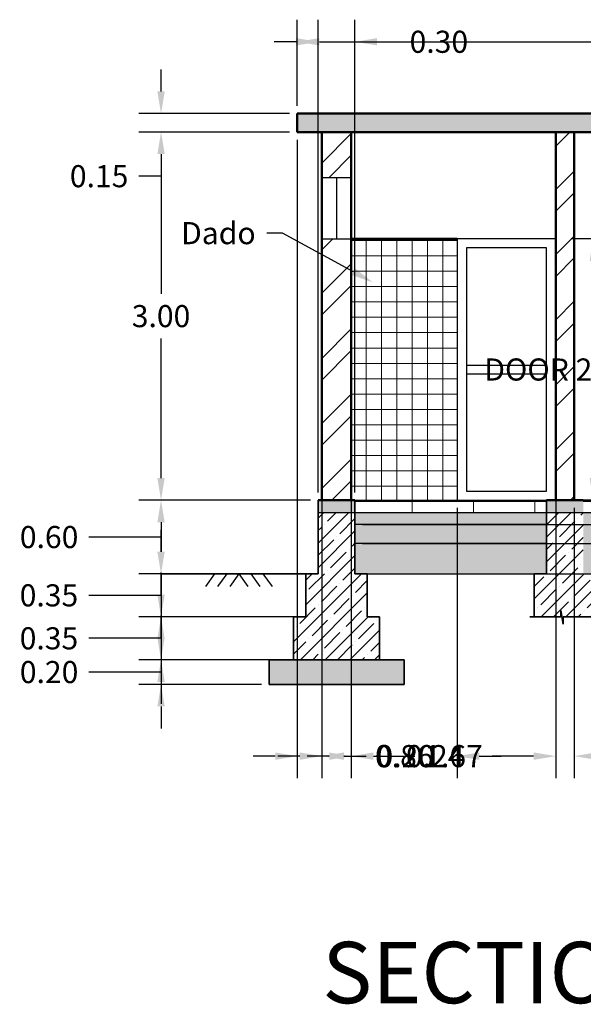
# Model space of a CAD drawing. Units: metres. Extents: x 22.1 to 34.4, y 4.4 to 12.4.
# Tile 1 of 8: x 22.1 to 26.6, y 4.4 to 12.4. Entities that reach past the tile are written whole.
import ezdxf
from ezdxf import colors
from ezdxf.entities.mleader import LeaderData, LeaderLine
from ezdxf.math import Vec2, Vec3

# ---------------------------------------------------------------- set-up
doc = ezdxf.new("R2010")
doc.units = ezdxf.units.M
doc.header["$MEASUREMENT"] = 0
for name, color, linetype, lineweight in [('A-ANNO-DIMS', 2, 'Continuous', 18), ('A-ANNO-TEXT', 7, 'Continuous', 18), ('A-DOOR', 4, 'Continuous', 25), ('A-FLOR', 3, 'Continuous', 25), ('A-FLOR-PATT', 252, 'Continuous', 13), ('A-GLAZ', 4, 'Continuous', 25), ('A-WALL', 7, 'Continuous', 50), ('A-WALL-PATT', 8, 'Continuous', 18), ('C-TOPO', 3, 'Continuous', 25), ('S-FNDN', 1, 'Continuous', 35), ('S-FNDN-PATT', 8, 'Continuous', 13), ('S-SLAB', 1, 'Continuous', 50), ('S-SLAB-PATT', 8, 'Continuous', 13)]:
    doc.layers.add(name, color=color, linetype=linetype, lineweight=lineweight)
doc.styles.get("Standard").update_dxf_attribs({"font": 'arial.ttf'})
doc.dimstyles.get("Standard").update_dxf_attribs({"dimtxt": 0.18, "dimasz": 0.18, "dimexe": 0.18, "dimexo": 0.0625, "dimgap": 0.09, "dimtad": 0, "dimtih": 1, "dimtoh": 1, "dimzin": 0, "dimdsep": 46, "dimtxsty": 'Standard', "dimcen": 0.09, "dimadec": 0, "dimazin": 0, "dimtfac": 1, "dimtofl": 0, "dimtmove": 0, "dimatfit": 3, "dimfxl": 1, "dimtolj": 1, "dimtzin": 0, "dimarcsym": 0})

# ---------------------------------------------------------------- blocks, each defined once
blk = doc.blocks.new('*D1')
at = {"layer": 'A-ANNO-DIMS', "color": 0, "lineweight": -2, "transparency": 16777216}
for p, q in [((23.2043, 11.8399), (23.2043, 12.0199)), ((24.2524, 11.6599), (23.0243, 11.6599)), ((24.2524, 11.5099), (23.0243, 11.5099)), ((23.2043, 11.3299), (23.2043, 11.1499)), ((23.2043, 11.1499), (23.0243, 11.1499))]:
    blk.add_line(p, q, dxfattribs=at)
at = {"layer": 'A-ANNO-DIMS', "color": 0, "transparency": 16777216}
for points in [[(23.1743, 11.8399), (23.2343, 11.8399), (23.2043, 11.6599)], [(23.1743, 11.3299), (23.2343, 11.3299), (23.2043, 11.5099)]]:
    blk.add_solid(points, dxfattribs=at)
at = {"layer": 'Defpoints', "color": 0, "transparency": 16777216}
for p in [(24.3149, 11.6599), (23.2043, 11.5099), (24.3149, 11.5099)]:
    blk.add_point(p, dxfattribs=at)
at = {"layer": 'A-ANNO-DIMS', "color": 0, "transparency": 16777216, "insert": (22.6998, 11.1499), "char_height": 0.18, "attachment_point": 5}
blk.add_mtext('\\A1;0.15', dxfattribs=at)
blk = doc.blocks.new('*D2')
at = {"layer": 'A-ANNO-DIMS', "color": 0, "lineweight": -2, "transparency": 16777216}
for p, q in [((24.2524, 11.5099), (23.0243, 11.5099)), ((23.2043, 11.3299), (23.2043, 10.1919)), ((23.2043, 8.6899), (23.2043, 9.8279)), ((24.4224, 8.5099), (23.0243, 8.5099))]:
    blk.add_line(p, q, dxfattribs=at)
at = {"layer": 'A-ANNO-DIMS', "color": 0, "transparency": 16777216}
for points in [[(23.1743, 11.3299), (23.2343, 11.3299), (23.2043, 11.5099)], [(23.1743, 8.6899), (23.2343, 8.6899), (23.2043, 8.5099)]]:
    blk.add_solid(points, dxfattribs=at)
at = {"layer": 'Defpoints', "color": 0, "transparency": 16777216}
for p in [(24.3149, 11.5099), (23.2043, 8.5099), (24.4849, 8.5099)]:
    blk.add_point(p, dxfattribs=at)
at = {"layer": 'A-ANNO-DIMS', "color": 0, "transparency": 16777216, "insert": (23.2043, 10.0099), "char_height": 0.18, "attachment_point": 5}
blk.add_mtext('\\A1;3.00', dxfattribs=at)
blk = doc.blocks.new('*D3')
at = {"layer": 'A-ANNO-DIMS', "color": 0, "lineweight": -2, "transparency": 16777216}
for p, q in [((24.4224, 8.5099), (23.0243, 8.5099)), ((23.2043, 8.3299), (23.2043, 8.0899)), ((22.7955, 8.2099), (22.6155, 8.2099)), ((23.2043, 8.2099), (22.7955, 8.2099)), ((24.4224, 7.9099), (23.0243, 7.9099))]:
    blk.add_line(p, q, dxfattribs=at)
at = {"layer": 'A-ANNO-DIMS', "color": 0, "transparency": 16777216}
for points in [[(23.1743, 8.3299), (23.2343, 8.3299), (23.2043, 8.5099)], [(23.1743, 8.0899), (23.2343, 8.0899), (23.2043, 7.9099)]]:
    blk.add_solid(points, dxfattribs=at)
at = {"layer": 'Defpoints', "color": 0, "transparency": 16777216}
for p in [(24.4849, 8.5099), (23.2043, 7.9099), (24.4849, 7.9099)]:
    blk.add_point(p, dxfattribs=at)
at = {"layer": 'A-ANNO-DIMS', "color": 0, "transparency": 16777216, "insert": (22.292, 8.2099), "char_height": 0.18, "attachment_point": 5}
blk.add_mtext('\\A1;0.60', dxfattribs=at)
blk = doc.blocks.new('*D4')
at = {"layer": 'A-ANNO-DIMS', "color": 0, "lineweight": -2, "transparency": 16777216}
for p, q in [((23.2043, 8.0899), (23.2043, 8.2699)), ((24.4224, 7.9099), (23.0243, 7.9099)), ((23.2043, 7.9099), (23.2043, 7.5599)), ((22.7954, 7.7349), (22.6154, 7.7349)), ((23.2043, 7.7349), (22.7954, 7.7349)), ((24.3224, 7.5599), (23.0243, 7.5599)), ((23.2043, 7.3799), (23.2043, 7.1999))]:
    blk.add_line(p, q, dxfattribs=at)
at = {"layer": 'A-ANNO-DIMS', "color": 0, "transparency": 16777216}
for points in [[(23.1743, 8.0899), (23.2343, 8.0899), (23.2043, 7.9099)], [(23.1743, 7.3799), (23.2343, 7.3799), (23.2043, 7.5599)]]:
    blk.add_solid(points, dxfattribs=at)
at = {"layer": 'Defpoints', "color": 0, "transparency": 16777216}
for p in [(24.4849, 7.9099), (23.2043, 7.5599), (24.3849, 7.5599)]:
    blk.add_point(p, dxfattribs=at)
at = {"layer": 'A-ANNO-DIMS', "color": 0, "transparency": 16777216, "insert": (22.2909, 7.7349), "char_height": 0.18, "attachment_point": 5}
blk.add_mtext('\\A1;0.35', dxfattribs=at)
blk = doc.blocks.new('*D5')
at = {"layer": 'A-ANNO-DIMS', "color": 0, "lineweight": -2, "transparency": 16777216}
for p, q in [((23.2043, 7.7399), (23.2043, 7.9199)), ((24.3224, 7.5599), (23.0243, 7.5599)), ((23.2043, 7.5599), (23.2043, 7.2099)), ((22.7954, 7.3849), (22.6154, 7.3849)), ((23.2043, 7.3849), (22.7954, 7.3849)), ((24.2224, 7.2099), (23.0243, 7.2099)), ((23.2043, 7.0299), (23.2043, 6.8499))]:
    blk.add_line(p, q, dxfattribs=at)
at = {"layer": 'A-ANNO-DIMS', "color": 0, "transparency": 16777216}
for points in [[(23.1743, 7.7399), (23.2343, 7.7399), (23.2043, 7.5599)], [(23.1743, 7.0299), (23.2343, 7.0299), (23.2043, 7.2099)]]:
    blk.add_solid(points, dxfattribs=at)
at = {"layer": 'Defpoints', "color": 0, "transparency": 16777216}
for p in [(24.3849, 7.5599), (23.2043, 7.2099), (24.2849, 7.2099)]:
    blk.add_point(p, dxfattribs=at)
at = {"layer": 'A-ANNO-DIMS', "color": 0, "transparency": 16777216, "insert": (22.2909, 7.3849), "char_height": 0.18, "attachment_point": 5}
blk.add_mtext('\\A1;0.35', dxfattribs=at)
blk = doc.blocks.new('*D6')
at = {"layer": 'A-ANNO-DIMS', "color": 0, "lineweight": -2, "transparency": 16777216}
for p, q in [((23.2043, 7.3899), (23.2043, 7.5699)), ((24.2224, 7.2099), (23.0243, 7.2099)), ((23.2043, 7.2099), (23.2043, 7.0099)), ((22.7955, 7.1099), (22.6155, 7.1099)), ((23.2043, 7.1099), (22.7955, 7.1099)), ((24.0224, 7.0099), (23.0243, 7.0099)), ((23.2043, 6.8299), (23.2043, 6.6499))]:
    blk.add_line(p, q, dxfattribs=at)
at = {"layer": 'A-ANNO-DIMS', "color": 0, "transparency": 16777216}
for points in [[(23.1743, 7.3899), (23.2343, 7.3899), (23.2043, 7.2099)], [(23.1743, 6.8299), (23.2343, 6.8299), (23.2043, 7.0099)]]:
    blk.add_solid(points, dxfattribs=at)
at = {"layer": 'Defpoints', "color": 0, "transparency": 16777216}
for p in [(24.2849, 7.2099), (23.2043, 7.0099), (24.0849, 7.0099)]:
    blk.add_point(p, dxfattribs=at)
at = {"layer": 'A-ANNO-DIMS', "color": 0, "transparency": 16777216, "insert": (22.292, 7.1099), "char_height": 0.18, "attachment_point": 5}
blk.add_mtext('\\A1;0.20', dxfattribs=at)
blk = doc.blocks.new('DOOR-800')
for p, q in [((26.4206, 10.6399), (25.6173, 10.6399)), ((25.6173, 10.6399), (25.6173, 8.5099)), ((26.4206, 8.5099), (26.4206, 10.6399)), ((25.6923, 10.5649), (25.6923, 8.5849)), ((26.3456, 10.5649), (25.6923, 10.5649)), ((26.3456, 8.5849), (26.3456, 10.5649)), ((25.6923, 9.6099), (26.3456, 9.6099)), ((25.6923, 9.5399), (26.3456, 9.5399)), ((25.6923, 8.5849), (26.3456, 8.5849)), ((25.6173, 8.5099), (26.4206, 8.5099))]:
    blk.add_line(p, q)
blk = doc.blocks.new('GROUND-SYMBOL')
for p, q in [((32.2587, 7.9099), (32.1846, 7.8067)), ((32.3571, 7.9099), (32.2831, 7.8067)), ((32.4556, 7.9099), (32.3816, 7.8067)), ((32.4556, 7.9099), (32.5296, 7.8067)), ((32.5541, 7.9099), (32.6281, 7.8067)), ((32.6525, 7.9099), (32.7266, 7.8067))]:
    blk.add_line(p, q)
blk = doc.blocks.new('*D16')
at = {"layer": 'A-ANNO-DIMS', "color": 0, "lineweight": -2, "transparency": 16777216}
for p, q in [((26.9843, 10.6399), (26.5473, 10.6399)), ((26.7273, 10.4599), (26.7273, 9.7581)), ((26.7273, 8.6899), (26.7273, 9.3917)), ((26.9843, 8.5099), (26.5473, 8.5099))]:
    blk.add_line(p, q, dxfattribs=at)
at = {"layer": 'A-ANNO-DIMS', "color": 0, "transparency": 16777216}
for points in [[(26.6973, 10.4599), (26.7573, 10.4599), (26.7273, 10.6399)], [(26.6973, 8.6899), (26.7573, 8.6899), (26.7273, 8.5099)]]:
    blk.add_solid(points, dxfattribs=at)
at = {"layer": 'Defpoints', "color": 0, "transparency": 16777216}
for p in [(26.7273, 10.6399), (27.0468, 10.6399), (27.0468, 8.5099)]:
    blk.add_point(p, dxfattribs=at)
at = {"layer": 'A-ANNO-DIMS', "color": 0, "transparency": 16777216, "insert": (26.7273, 9.5749), "char_height": 0.18, "attachment_point": 5}
blk.add_mtext('\\A1;DOOR 2.13 TYP.', dxfattribs=at)
blk = doc.blocks.new('*D22')
at = {"layer": 'A-ANNO-DIMS', "color": 0, "lineweight": -2, "transparency": 16777216}
for p, q in [((24.7549, 11.4474), (24.7549, 6.2449)), ((26.4206, 11.4474), (26.4206, 6.2449)), ((24.9349, 6.4249), (25.2724, 6.4249)), ((26.2406, 6.4249), (25.903, 6.4249))]:
    blk.add_line(p, q, dxfattribs=at)
at = {"layer": 'A-ANNO-DIMS', "color": 0, "transparency": 16777216}
for points in [[(24.9349, 6.4549), (24.9349, 6.3949), (24.7549, 6.4249)], [(26.2406, 6.4549), (26.2406, 6.3949), (26.4206, 6.4249)]]:
    blk.add_solid(points, dxfattribs=at)
at = {"layer": 'Defpoints', "color": 0, "transparency": 16777216}
for p in [(24.7549, 11.5099), (26.4206, 11.5099), (26.4206, 6.4249)]:
    blk.add_point(p, dxfattribs=at)
at = {"layer": 'A-ANNO-DIMS', "color": 0, "transparency": 16777216, "insert": (25.5877, 6.4249), "char_height": 0.18, "attachment_point": 5}
blk.add_mtext('\\A1;1.67', dxfattribs=at)
blk = doc.blocks.new('*D24')
at = {"layer": 'A-ANNO-DIMS', "color": 0, "lineweight": -2, "transparency": 16777216}
for p, q in [((24.3149, 11.4474), (24.3149, 6.2449)), ((24.5149, 11.4474), (24.5149, 6.2449)), ((24.1349, 6.4249), (23.9549, 6.4249)), ((24.6949, 6.4249), (24.8749, 6.4249))]:
    blk.add_line(p, q, dxfattribs=at)
at = {"layer": 'A-ANNO-DIMS', "color": 0, "transparency": 16777216}
for points in [[(24.1349, 6.4549), (24.1349, 6.3949), (24.3149, 6.4249)], [(24.6949, 6.4549), (24.6949, 6.3949), (24.5149, 6.4249)]]:
    blk.add_solid(points, dxfattribs=at)
at = {"layer": 'Defpoints', "color": 0, "transparency": 16777216}
for p in [(24.3149, 11.5099), (24.5149, 11.5099), (24.5149, 6.4249)]:
    blk.add_point(p, dxfattribs=at)
at = {"layer": 'A-ANNO-DIMS', "color": 0, "transparency": 16777216, "insert": (25.1984, 6.4249), "char_height": 0.18, "attachment_point": 5}
blk.add_mtext('\\A1;0.20', dxfattribs=at)
blk = doc.blocks.new('*D25')
at = {"layer": 'A-ANNO-DIMS', "color": 0, "lineweight": -2, "transparency": 16777216}
for p, q in [((24.5149, 11.4474), (24.5149, 6.2449)), ((24.7549, 11.4474), (24.7549, 6.2449)), ((24.3349, 6.4249), (24.1549, 6.4249)), ((24.9349, 6.4249), (25.1149, 6.4249))]:
    blk.add_line(p, q, dxfattribs=at)
at = {"layer": 'A-ANNO-DIMS', "color": 0, "transparency": 16777216}
for points in [[(24.3349, 6.4549), (24.3349, 6.3949), (24.5149, 6.4249)], [(24.9349, 6.4549), (24.9349, 6.3949), (24.7549, 6.4249)]]:
    blk.add_solid(points, dxfattribs=at)
at = {"layer": 'Defpoints', "color": 0, "transparency": 16777216}
for p in [(24.5149, 11.5099), (24.7549, 11.5099), (24.7549, 6.4249)]:
    blk.add_point(p, dxfattribs=at)
at = {"layer": 'A-ANNO-DIMS', "color": 0, "transparency": 16777216, "insert": (25.4383, 6.4249), "char_height": 0.18, "attachment_point": 5}
blk.add_mtext('\\A1;0.24', dxfattribs=at)
blk = doc.blocks.new('*D29')
at = {"layer": 'A-ANNO-DIMS', "color": 0, "lineweight": -2, "transparency": 16777216}
for p, q in [((24.3149, 11.7224), (24.3149, 12.4249)), ((31.9781, 11.7224), (31.9781, 12.4249)), ((24.4949, 12.2449), (27.7535, 12.2449)), ((31.7981, 12.2449), (28.5394, 12.2449))]:
    blk.add_line(p, q, dxfattribs=at)
at = {"layer": 'A-ANNO-DIMS', "color": 0, "transparency": 16777216}
for points in [[(24.4949, 12.2749), (24.4949, 12.2149), (24.3149, 12.2449)], [(31.7981, 12.2749), (31.7981, 12.2149), (31.9781, 12.2449)]]:
    blk.add_solid(points, dxfattribs=at)
at = {"layer": 'Defpoints', "color": 0, "transparency": 16777216}
for p in [(31.9781, 12.2449), (24.3149, 11.6599), (31.9781, 11.6599)]:
    blk.add_point(p, dxfattribs=at)
at = {"layer": 'A-ANNO-DIMS', "color": 0, "transparency": 16777216, "insert": (28.1465, 12.2449), "char_height": 0.18, "attachment_point": 5}
blk.add_mtext('\\A1;7.663', dxfattribs=at)
blk = doc.blocks.new('*D30')
at = {"layer": 'A-ANNO-DIMS', "color": 0, "lineweight": -2, "transparency": 16777216}
for p, q in [((24.7549, 8.4474), (24.7549, 6.2449)), ((25.6173, 8.4474), (25.6173, 6.2449)), ((24.5749, 6.4249), (24.3949, 6.4249)), ((25.7973, 6.4249), (25.9773, 6.4249))]:
    blk.add_line(p, q, dxfattribs=at)
at = {"layer": 'A-ANNO-DIMS', "color": 0, "transparency": 16777216}
for points in [[(24.5749, 6.4549), (24.5749, 6.3949), (24.7549, 6.4249)], [(25.7973, 6.4549), (25.7973, 6.3949), (25.6173, 6.4249)]]:
    blk.add_solid(points, dxfattribs=at)
at = {"layer": 'Defpoints', "color": 0, "transparency": 16777216}
for p in [(24.7549, 8.5099), (25.6173, 8.5099), (25.6173, 6.4249)]:
    blk.add_point(p, dxfattribs=at)
at = {"layer": 'A-ANNO-DIMS', "color": 0, "transparency": 16777216, "insert": (25.1861, 6.4249), "char_height": 0.18, "attachment_point": 5}
blk.add_mtext('\\A1;0.86', dxfattribs=at)
blk = doc.blocks.new('*D31')
at = {"layer": 'A-ANNO-DIMS', "color": 0, "lineweight": -2, "transparency": 16777216}
for p, q in [((26.4206, 8.4474), (26.4206, 6.2449)), ((26.5706, 8.4474), (26.5706, 6.2449)), ((26.2406, 6.4249), (26.0606, 6.4249)), ((26.7506, 6.4249), (26.9306, 6.4249))]:
    blk.add_line(p, q, dxfattribs=at)
at = {"layer": 'A-ANNO-DIMS', "color": 0, "transparency": 16777216}
for points in [[(26.2406, 6.4549), (26.2406, 6.3949), (26.4206, 6.4249)], [(26.7506, 6.4549), (26.7506, 6.3949), (26.5706, 6.4249)]]:
    blk.add_solid(points, dxfattribs=at)
at = {"layer": 'Defpoints', "color": 0, "transparency": 16777216}
for p in [(26.4206, 8.5099), (26.5706, 8.5099), (26.5706, 6.4249)]:
    blk.add_point(p, dxfattribs=at)
at = {"layer": 'A-ANNO-DIMS', "color": 0, "transparency": 16777216, "insert": (27.255, 6.4249), "char_height": 0.18, "attachment_point": 5}
blk.add_mtext('\\A1;0.15', dxfattribs=at)
blk = doc.blocks.new('*D32')
at = {"layer": 'A-ANNO-DIMS', "color": 0, "lineweight": -2, "transparency": 16777216}
for p, q in [((26.5706, 8.4474), (26.5706, 6.2449)), ((27.8501, 8.4474), (27.8501, 6.2449)), ((26.7506, 6.4249), (26.8948, 6.4249)), ((27.6701, 6.4249), (27.5258, 6.4249))]:
    blk.add_line(p, q, dxfattribs=at)
at = {"layer": 'A-ANNO-DIMS', "color": 0, "transparency": 16777216}
for points in [[(26.7506, 6.4549), (26.7506, 6.3949), (26.5706, 6.4249)], [(27.6701, 6.4549), (27.6701, 6.3949), (27.8501, 6.4249)]]:
    blk.add_solid(points, dxfattribs=at)
at = {"layer": 'Defpoints', "color": 0, "transparency": 16777216}
for p in [(26.5706, 8.5099), (27.8501, 8.5099), (27.8501, 6.4249)]:
    blk.add_point(p, dxfattribs=at)
at = {"layer": 'A-ANNO-DIMS', "color": 0, "transparency": 16777216, "insert": (27.2103, 6.4249), "char_height": 0.18, "attachment_point": 5}
blk.add_mtext('\\A1;1.28', dxfattribs=at)
blk = doc.blocks.new('*D44')
at = {"layer": 'A-ANNO-DIMS', "color": 0, "lineweight": -2, "transparency": 16777216}
for p, q in [((33.6737, 8.6899), (33.6737, 8.8699)), ((24.8474, 8.5099), (33.8537, 8.5099)), ((24.5474, 8.4099), (33.8537, 8.4099)), ((33.6737, 8.2299), (33.6737, 8.0499)), ((33.6737, 8.0499), (33.4937, 8.0499))]:
    blk.add_line(p, q, dxfattribs=at)
at = {"layer": 'A-ANNO-DIMS', "color": 0, "transparency": 16777216}
for points in [[(33.6437, 8.6899), (33.7037, 8.6899), (33.6737, 8.5099)], [(33.6437, 8.2299), (33.7037, 8.2299), (33.6737, 8.4099)]]:
    blk.add_solid(points, dxfattribs=at)
at = {"layer": 'Defpoints', "color": 0, "transparency": 16777216}
for p in [(24.7849, 8.5099), (24.4849, 8.4099), (33.6737, 8.4099)]:
    blk.add_point(p, dxfattribs=at)
at = {"layer": 'A-ANNO-DIMS', "color": 0, "transparency": 16777216, "insert": (33.1702, 8.0499), "char_height": 0.18, "attachment_point": 5}
blk.add_mtext('\\A1;0.10', dxfattribs=at)
blk = doc.blocks.new('*D45')
at = {"layer": 'A-ANNO-DIMS', "color": 0, "lineweight": -2, "transparency": 16777216}
for p, q in [((33.6737, 8.5899), (33.6737, 8.7699)), ((24.5474, 8.4099), (33.8537, 8.4099)), ((24.8474, 8.3119), (33.8537, 8.3119)), ((33.6737, 8.1319), (33.6737, 7.9519)), ((33.6737, 7.9519), (33.4937, 7.9519))]:
    blk.add_line(p, q, dxfattribs=at)
at = {"layer": 'A-ANNO-DIMS', "color": 0, "transparency": 16777216}
for points in [[(33.6437, 8.5899), (33.7037, 8.5899), (33.6737, 8.4099)], [(33.6437, 8.1319), (33.7037, 8.1319), (33.6737, 8.3119)]]:
    blk.add_solid(points, dxfattribs=at)
at = {"layer": 'Defpoints', "color": 0, "transparency": 16777216}
for p in [(24.4849, 8.4099), (24.7849, 8.3119), (33.6737, 8.3119)]:
    blk.add_point(p, dxfattribs=at)
at = {"layer": 'A-ANNO-DIMS', "color": 0, "transparency": 16777216, "insert": (33.0998, 7.9519), "char_height": 0.18, "attachment_point": 5}
blk.add_mtext('\\A1;0.098', dxfattribs=at)
blk = doc.blocks.new('*D46')
at = {"layer": 'A-ANNO-DIMS', "color": 0, "lineweight": -2, "transparency": 16777216}
for p, q in [((33.6737, 8.4919), (33.6737, 8.6719)), ((24.8474, 8.3119), (33.8537, 8.3119)), ((24.8474, 8.1578), (33.8537, 8.1578)), ((33.6737, 7.9778), (33.6737, 7.7978)), ((33.6737, 7.7978), (33.4937, 7.7978))]:
    blk.add_line(p, q, dxfattribs=at)
at = {"layer": 'A-ANNO-DIMS', "color": 0, "transparency": 16777216}
for points in [[(33.6437, 8.4919), (33.7037, 8.4919), (33.6737, 8.3119)], [(33.6437, 7.9778), (33.7037, 7.9778), (33.6737, 8.1578)]]:
    blk.add_solid(points, dxfattribs=at)
at = {"layer": 'Defpoints', "color": 0, "transparency": 16777216}
for p in [(24.7849, 8.3119), (24.7849, 8.1578), (33.6737, 8.1578)]:
    blk.add_point(p, dxfattribs=at)
at = {"layer": 'A-ANNO-DIMS', "color": 0, "transparency": 16777216, "insert": (33.1692, 7.7978), "char_height": 0.18, "attachment_point": 5}
blk.add_mtext('\\A1;0.15', dxfattribs=at)
blk = doc.blocks.new('*D47')
at = {"layer": 'A-ANNO-DIMS', "color": 0, "lineweight": -2, "transparency": 16777216}
for p, q in [((33.6737, 8.3378), (33.6737, 8.5178)), ((24.8474, 8.1578), (33.8537, 8.1578)), ((24.8474, 7.9099), (33.8537, 7.9099)), ((33.6737, 7.7299), (33.6737, 7.5499)), ((33.6737, 7.5499), (33.4937, 7.5499))]:
    blk.add_line(p, q, dxfattribs=at)
at = {"layer": 'A-ANNO-DIMS', "color": 0, "transparency": 16777216}
for points in [[(33.6437, 8.3378), (33.7037, 8.3378), (33.6737, 8.1578)], [(33.6437, 7.7299), (33.7037, 7.7299), (33.6737, 7.9099)]]:
    blk.add_solid(points, dxfattribs=at)
at = {"layer": 'Defpoints', "color": 0, "transparency": 16777216}
for p in [(24.7849, 8.1578), (24.7849, 7.9099), (33.6737, 7.9099)]:
    blk.add_point(p, dxfattribs=at)
at = {"layer": 'A-ANNO-DIMS', "color": 0, "transparency": 16777216, "insert": (33.1692, 7.5499), "char_height": 0.18, "attachment_point": 5}
blk.add_mtext('\\A1;0.25', dxfattribs=at)
blk = doc.blocks.new('*D48')
at = {"layer": 'A-ANNO-DIMS', "color": 0, "lineweight": -2, "transparency": 16777216}
for p, q in [((24.4849, 8.5724), (24.4849, 12.4249)), ((24.7849, 8.5724), (24.7849, 12.4249)), ((24.3049, 12.2449), (24.1249, 12.2449)), ((24.9649, 12.2449), (25.1449, 12.2449))]:
    blk.add_line(p, q, dxfattribs=at)
at = {"layer": 'A-ANNO-DIMS', "color": 0, "transparency": 16777216}
for points in [[(24.3049, 12.2749), (24.3049, 12.2149), (24.4849, 12.2449)], [(24.9649, 12.2749), (24.9649, 12.2149), (24.7849, 12.2449)]]:
    blk.add_solid(points, dxfattribs=at)
at = {"layer": 'Defpoints', "color": 0, "transparency": 16777216}
for p in [(24.7849, 12.2449), (24.4849, 8.5099), (24.7849, 8.5099)]:
    blk.add_point(p, dxfattribs=at)
at = {"layer": 'A-ANNO-DIMS', "color": 0, "transparency": 16777216, "insert": (25.4684, 12.2449), "char_height": 0.18, "attachment_point": 5}
blk.add_mtext('\\A1;0.30', dxfattribs=at)

msp = doc.modelspace()

# ---------------------------------------------------------------- hatches: boundary and pattern name
at = {"layer": 'A-FLOR-PATT'}
h = msp.add_hatch(dxfattribs=at)
h.set_pattern_fill('BRICK', color=256)
h.paths.add_polyline_path([(31.5081, 8.5099), (28.1201, 8.5099), (28.1201, 8.4099), (31.5081, 8.4099)])
h.paths.add_polyline_path([(27.8201, 8.5099), (27.0468, 8.5099), (26.6456, 8.5099), (26.6456, 8.4099), (27.8201, 8.4099)])
h.paths.add_polyline_path([(26.3456, 8.5099), (25.6173, 8.5099), (24.7849, 8.5099), (24.7849, 8.4099), (26.3456, 8.4099)])
h = msp.add_hatch(dxfattribs=at)
h.set_pattern_fill('AR-SAND', color=256, scale=0.57)
h.paths.add_polyline_path([(26.3456, 8.4099), (24.7849, 8.4099), (24.7849, 8.3119), (26.3456, 8.3119)])
h.paths.add_polyline_path([(27.8201, 8.4099), (26.6456, 8.4099), (26.6456, 8.3119), (27.8201, 8.3119)])
h.paths.add_polyline_path([(31.5081, 8.4099), (28.1201, 8.4099), (28.1201, 8.3119), (31.5081, 8.3119)])
h = msp.add_hatch(dxfattribs=at)
h.set_pattern_fill('AR-SAND', color=256, scale=0.57)
h.paths.add_polyline_path([(31.5081, 8.4099), (28.1201, 8.4099), (28.1201, 8.3119), (31.5081, 8.3119)])
h.paths.add_polyline_path([(27.8201, 8.4099), (26.6456, 8.4099), (26.6456, 8.3119), (27.8201, 8.3119)])
h.paths.add_polyline_path([(26.3456, 8.4099), (24.7849, 8.4099), (24.7849, 8.3119), (26.3456, 8.3119)])
h = msp.add_hatch(dxfattribs=at)
h.set_pattern_fill('AR-SAND', color=256, scale=0.04)
h.paths.add_polyline_path([(26.3456, 8.4099), (24.7849, 8.4099), (24.7849, 8.3119), (26.3456, 8.3119)])
h.paths.add_polyline_path([(27.8201, 8.4099), (26.6456, 8.4099), (26.6456, 8.3119), (27.8201, 8.3119)])
h.paths.add_polyline_path([(31.5081, 8.4099), (28.1201, 8.4099), (28.1201, 8.3119), (31.5081, 8.3119)])
h = msp.add_hatch(dxfattribs=at)
h.set_pattern_fill('GRAVEL', color=256, scale=0.18)
h.set_pattern_definition([(228.012788, (0.1296, 0.18), (-1.44, -1.62), [0.0242165, -2.39743585]), (184.96974, (0.1134, 0.162), (2.16, 0.18), [0.0415562, -4.1140665]), (132.510447, (0.072, 0.1584), (1.8, -1.98), [0.0293018, -2.9008859]), (267.27369, (0.0018, 0.1134), (0.18, 3.6), [0.0378428, -3.74644045]), (292.833654, (0, 0.0756), (-0.9, 2.16), [0.0371079, -3.6736872]), (357.27369, (0.0144, 0.0414), (-3.6, 0.18), [0.0378428, -3.74644045]), (37.69424, (0.0522, 0.0396), (-2.34, -1.8), [0.0500452, -4.9544727]), (72.255328, (0.0918, 0.0702), (1.26, 3.96), [0.0472478, -4.6775379]), (121.429566, (0.1062, 0.1152), (-1.44, 2.34), [0.037971, -3.7591332]), (175.23636, (0.0864, 0.1476), (1.98, -0.18), [0.0433498, -2.1241373]), (222.397438, (0.0432, 0.1512), (-2.16, -1.98), [0.0560606, -5.5500075]), (138.814075, (0.18, 0.1116), (-1.26, 1.08), [0.0191342, -1.8942921]), (171.469234, (0.1656, 0.1242), (2.34, -0.36), [0.0364027, -3.60387205]), (225, (0.1296, 0.1296), (0, -0.18), [0.0254558, -0.2291027]), (203.19859, (0.117, 0.1512), (0.9, 0.36), [0.0137084, -1.3571307]), (291.80141, (0.1044, 0.1458), (-0.18, 0.54), [0.0193865, -0.9499431]), (30.96376, (0.1116, 0.1278), (0.54, 0.36), [0.0314872, -1.0180841]), (161.56505, (0.1386, 0.144), (0.36, -0.18), [0.0227684, -0.5464416]), (16.38954, (0, 0.1458), (1.8, 0.54), [0.031896, -3.1577121]), (70.346176, (0.0306, 0.1548), (-0.72, -1.98), [0.026759, -2.6491334]), (293.19859, (0.1386, 0.18), (-0.36, 0.9), [0.0274167, -1.3434225]), (343.61046, (0.1494, 0.1548), (-1.8, 0.54), [0.031896, -3.1577121]), (339.443955, (0, 0.0342), (-0.9, 0.36), [0.0307584, -1.5071623]), (294.77514, (0.0288, 0.0234), (-0.9, 1.98), [0.025772, -2.55143575]), (66.80141, (0.1404, 0), (0.36, 0.9), [0.0274167, -1.3434225]), (17.354025, (0.1512, 0.0252), (-2.34, -0.72), [0.0301736, -2.98717625]), (69.443955, (0.0522, 0), (-0.36, -0.9), [0.0153792, -1.5225415]), (101.30993, (0.1296, 0), (-0.18, 0.72), [0.0091782, -0.9086453]), (165.96376, (0.1278, 0.009), (0.54, -0.18), [0.0371079, -0.7050511]), (186.009006, (0.0918, 0.018), (1.8, 0.18), [0.034389, -3.4045062]), (303.69007, (0.1116, 0.1116), (-0.18, 0.36), [0.02596, -0.6230393]), (353.157227, (0.126, 0.09), (3.06, -0.36), [0.0453229, -4.4869613]), (60.945396, (0.171, 0.0846), (-0.72, -1.26), [0.0185321, -1.8346813]), (90, (0.18, 0.1008), (-0.18, 0.18), [0.0108, -0.1692]), (120.256437, (0.0882, 0.0234), (0.72, -1.26), [0.0250063, -2.4756336]), (48.012788, (0.0756, 0.045), (1.44, 1.62), [0.048433, -2.3732194]), (0, (0.108, 0.081), (0.18, 0.18), [0.0468, -0.1332]), (325.304846, (0.1548, 0.081), (1.8, -1.26), [0.0284605, -2.8175894]), (254.0546, (0.1782, 0.0648), (-0.18, -0.72), [0.0262084, -1.2842114]), (207.645975, (0.171, 0.0396), (-3.42, -1.8), [0.0426717, -4.22450535]), (175.42608, (0.1332, 0.0198), (-2.34, 0.18), [0.0451438, -4.4692332])])
h.paths.add_polyline_path([(26.3456, 8.1578), (24.7849, 8.1578), (24.7849, 7.9099), (24.8849, 7.9099), (26.3456, 7.9099)])
h.paths.add_polyline_path([(27.8201, 8.1578), (26.6456, 8.1578), (26.6456, 7.9099), (26.7456, 7.9099), (27.8201, 7.9099)])
h.paths.add_polyline_path([(31.5081, 8.1578), (28.1201, 8.1578), (28.1201, 7.9099), (31.4081, 7.9099), (31.5081, 7.9099)])
at = {"layer": 'A-WALL-PATT'}
h = msp.add_hatch(dxfattribs=at)
h.set_pattern_fill('ANSI32', color=256)
h.paths.add_polyline_path([(24.7549, 11.5099), (24.5149, 11.5099), (24.5149, 11.1399), (24.7549, 11.1399)])
h.paths.add_polyline_path([(24.7549, 10.6399), (24.5149, 10.6399), (24.5149, 8.5099), (24.6349, 8.5099), (24.7549, 8.5099)])
h.paths.add_polyline_path([(26.5706, 11.5099), (26.4206, 11.5099), (26.4206, 8.5099), (26.5706, 8.5099)])
h.paths.add_polyline_path([(28.0901, 10.6399), (28.0901, 11.5099), (27.8501, 11.5099), (27.8501, 8.5099), (28.0901, 8.5099)])
h.paths.add_polyline_path([(31.7781, 11.5099), (31.5381, 11.5099), (31.5381, 8.5099), (31.6581, 8.5099), (31.7781, 8.5099)])
h = msp.add_hatch(dxfattribs=at)
h.set_pattern_fill('NET', color=256)
h.paths.add_polyline_path([(25.6173, 10.6399), (24.7549, 10.6399), (24.7549, 8.5099), (24.7849, 8.5099), (25.6173, 8.5099)])
at = {"layer": 'S-FNDN-PATT'}
h = msp.add_hatch(dxfattribs=at)
h.set_pattern_fill('ANSI35', color=256, scale=0.57)
h.paths.add_polyline_path([(24.3849, 7.5599), (24.2849, 7.5599), (24.2849, 7.2099), (24.9849, 7.2099), (24.9849, 7.5599), (24.8849, 7.5599), (24.8849, 7.9099), (24.7849, 7.9099), (24.7849, 8.4099), (24.4849, 8.4099), (24.4849, 7.9099), (24.3849, 7.9099)])
h.paths.add_polyline_path([(27.7201, 7.5599), (27.6201, 7.5599), (27.6201, 7.2099), (28.3201, 7.2099), (28.3201, 7.5599), (28.2201, 7.5599), (28.2201, 7.9099), (28.1201, 7.9099), (28.1201, 8.4099), (27.8201, 8.4099), (27.8201, 7.9099), (27.7201, 7.9099)])
h.paths.add_polyline_path([(26.7456, 7.9099), (26.6456, 7.9099), (26.6456, 8.4099), (26.3456, 8.4099), (26.3456, 7.9099), (26.2456, 7.9099), (26.2456, 7.5599), (26.4616, 7.5599), (26.4616, 7.6127), (26.4825, 7.5003), (26.4825, 7.5599), (26.7456, 7.5599)])
h.paths.add_polyline_path([(31.8581, 7.5599), (31.8581, 7.9099), (31.8081, 7.9099), (31.8081, 8.4099), (31.5081, 8.4099), (31.5081, 7.9099), (31.4581, 7.9099), (31.4581, 7.5599), (31.3581, 7.5599), (31.3581, 7.2099), (31.9581, 7.2099), (31.9581, 7.5599)])
at = {"layer": 'S-SLAB-PATT'}
h = msp.add_hatch(dxfattribs=at)
h.set_pattern_fill('AR-CONC', color=256, scale=0.04)
h.set_pattern_definition([(50, (0, 0), (0.286904, -0.0251009), [0.03, -0.33]), (355, (0, 0), (-0.0555005, 0.3008769), [0.024, -0.264]), (100.4514, (0.0239, -0.0021), (0.2314035, 0.275776), [0.025496, -0.2804568]), (46.1842, (0, 0.08), (0.4268965, -0.0662077), [0.045, -0.495]), (96.6356, (0.03557, 0.0745), (0.373865, 0.3896474), [0.038244, -0.4206855]), (351.1842, (0, 0.08), (0.373865, 0.3896474), [0.036, -0.396]), (21, (0.04, 0.06), (0.2387628, -0.1610476), [0.03, -0.33]), (326, (0.04, 0.06), (0.0973261, 0.29006), [0.024, -0.264]), (71.4514, (0.0599, 0.04658), (0.336089, 0.1290125), [0.025496, -0.2804568]), (37.5, (0, 0), (0.00486394, 0.13315754), [0, -0.2608, 0, -0.268, 0, -0.265]), (7.5, (0, 0), (0.1052278, 0.1577647), [0, -0.1528, 0, -0.2548, 0, -0.101]), (327.5, (-0.0892, 0), (0.21352897, -0.00902195), [0, -0.1, 0, -0.312, 0, -0.414]), (317.5, (-0.1292, 0), (0.2332745, 0.040042), [0, -0.13, 0, -0.2072, 0, -0.294])])
h.paths.add_polyline_path([(31.9781, 11.6599), (24.3149, 11.6599), (24.3149, 11.5099), (24.5149, 11.5099), (31.7781, 11.5099), (31.9781, 11.5099)])
h.paths.add_polyline_path([(25.1849, 7.2099), (24.9849, 7.2099), (24.0849, 7.2099), (24.0849, 7.0099), (25.1849, 7.0099)])
h.paths.add_polyline_path([(32.2081, 7.2099), (32.0081, 7.2099), (31.1081, 7.2099), (31.1081, 7.0099), (32.2081, 7.0099)])
h.paths.add_polyline_path([(28.5201, 7.2099), (28.3201, 7.2099), (27.4201, 7.2099), (27.4201, 7.0099), (28.5201, 7.0099)])
h.paths.add_polyline_path([(24.7849, 8.5099), (24.6349, 8.5099), (24.5149, 8.5099), (24.4849, 8.5099), (24.4849, 8.4099), (24.7849, 8.4099)])
h.paths.add_polyline_path([(26.6456, 8.5099), (26.3456, 8.5099), (26.3456, 8.4099), (26.6456, 8.4099)])
h.paths.add_polyline_path([(28.1201, 8.5099), (28.0901, 8.5099), (27.8201, 8.5099), (27.8201, 8.4099), (28.1201, 8.4099)])
h.paths.add_polyline_path([(31.8081, 8.5099), (31.6581, 8.5099), (31.5381, 8.5099), (31.5081, 8.5099), (31.5081, 8.4099), (31.8081, 8.4099)])
h.paths.add_polyline_path([(26.3456, 8.3119), (24.7849, 8.3119), (24.7849, 8.1578), (26.3456, 8.1578)])
h.paths.add_polyline_path([(27.8201, 8.3119), (26.6456, 8.3119), (26.6456, 8.1578), (27.8201, 8.1578)])
h.paths.add_polyline_path([(31.5081, 8.3119), (28.1201, 8.3119), (28.1201, 8.1578), (31.5081, 8.1578)])

# ---------------------------------------------------------------- linework, layer by layer
at = {"layer": 'A-FLOR'}
for p, q in [((24.7849, 8.5099), (31.5081, 8.5099)), ((24.4849, 8.4099), (26.6456, 8.4099)), ((26.3456, 8.3119), (24.7849, 8.3119)), ((26.3456, 8.1578), (24.7849, 8.1578)), ((24.8849, 7.9099), (26.3456, 7.9099))]:
    msp.add_line(p, q, dxfattribs=at)
at = {"layer": 'A-GLAZ'}
for p, q in [((24.5149, 11.1399), (24.7549, 11.1399)), ((24.6349, 11.1399), (24.6349, 10.6399)), ((24.5149, 10.6399), (24.7549, 10.6399))]:
    msp.add_line(p, q, dxfattribs=at)
at = {"layer": 'A-WALL'}
for p, q in [((24.5149, 8.5099), (24.5149, 11.5099)), ((24.5149, 11.5099), (24.6349, 11.5099)), ((24.7549, 11.5099), (24.6349, 11.5099)), ((24.7549, 8.5099), (24.7549, 11.5099)), ((26.4206, 8.5099), (26.4206, 11.5099)), ((26.4206, 11.5099), (26.5706, 11.5099)), ((26.5706, 11.5099), (26.5706, 8.5099)), ((25.6173, 10.6399), (24.7549, 10.6399)), ((24.4849, 8.5099), (24.6349, 8.5099)), ((24.6349, 8.5099), (24.5149, 8.5099)), ((24.7849, 8.5099), (24.6349, 8.5099)), ((24.6349, 8.5099), (24.7549, 8.5099)), ((26.3456, 8.5099), (26.6456, 8.5099))]:
    msp.add_line(p, q, dxfattribs=at)
at = {"layer": 'C-TOPO'}
msp.add_line((23.2043, 7.9099), (24.3849, 7.9099), dxfattribs=at)
at = {"layer": 'S-FNDN'}
for p, q in [((24.4849, 7.9099), (24.4849, 8.5099)), ((24.7849, 7.9099), (24.7849, 8.5099)), ((26.3456, 7.9099), (26.3456, 8.5099)), ((24.3849, 7.5599), (24.3849, 7.9099)), ((24.3849, 7.9099), (24.4849, 7.9099)), ((24.8849, 7.9099), (24.7849, 7.9099)), ((24.8849, 7.5599), (24.8849, 7.9099)), ((26.2456, 7.5599), (26.2456, 7.9099)), ((26.2456, 7.9099), (26.3456, 7.9099)), ((24.2849, 7.2099), (24.2849, 7.5599)), ((24.2849, 7.5599), (24.3849, 7.5599)), ((24.9849, 7.5599), (24.8849, 7.5599)), ((24.9849, 7.2099), (24.9849, 7.5599)), ((26.2456, 7.5599), (26.2103, 7.5599)), ((26.2456, 7.5599), (26.4616, 7.5599)), ((26.4616, 7.5599), (26.4616, 7.6127)), ((26.4616, 7.6127), (26.4825, 7.5003)), ((26.4825, 7.5003), (26.4825, 7.5599)), ((26.4825, 7.5599), (26.7961, 7.5599)), ((24.0849, 7.0099), (24.0849, 7.2099)), ((24.0849, 7.2099), (24.9849, 7.2099)), ((25.1849, 7.2099), (24.9849, 7.2099)), ((25.1849, 7.2099), (25.1849, 7.0099)), ((24.0849, 7.0099), (25.1849, 7.0099))]:
    msp.add_line(p, q, dxfattribs=at)
at = {"layer": 'S-SLAB'}
for p, q in [((31.9781, 11.6599), (24.3149, 11.6599)), ((24.3149, 11.5099), (24.3149, 11.6599)), ((24.5149, 11.5099), (24.3149, 11.5099)), ((24.5149, 11.5099), (31.7781, 11.5099))]:
    msp.add_line(p, q, dxfattribs=at)

# ---------------------------------------------------------------- block references
at = {"layer": 'A-DOOR'}
msp.add_blockref('DOOR-800', (0, 0), dxfattribs=at)
at = {"layer": 'C-TOPO'}
msp.add_blockref('GROUND-SYMBOL', (-8.6177, 0), dxfattribs=at)

# ---------------------------------------------------------------- texts
at = {"layer": 'A-ANNO-TEXT', "insert": (24.5182, 4.9119), "char_height": 0.5, "attachment_point": 1}
msp.add_mtext_dynamic_manual_height_columns('SECTION ABCD', width=6.025695, gutter_width=0.858, heights=[0], dxfattribs=at)

# ---------------------------------------------------------------- dimensions: what is measured, and where the dimension line sits
at = {"layer": 'A-ANNO-DIMS'}
for base, p1, p2, override, picture, middle in [((24.7849, 12.2449), (24.4849, 8.5099), (24.7849, 8.5099), {"dimdec": 2, "dimlfac": 1, "dimrnd": 0, "dimzin": 0, "dimdsep": 46, "dimlunit": 2}, '*D48', (25.4684, 12.2449)), ((31.9781, 12.2449), (24.3149, 11.6599), (31.9781, 11.6599), {"dimdec": 3, "dimlfac": 1, "dimrnd": 0, "dimzin": 0, "dimdsep": 46, "dimlunit": 2}, '*D29', (28.1465, 12.2449)), ((24.5149, 6.4249), (24.3149, 11.5099), (24.5149, 11.5099), {"dimdec": 2, "dimlfac": 1, "dimrnd": 0, "dimzin": 0, "dimdsep": 46, "dimlunit": 2}, '*D24', (25.1984, 6.4249)), ((24.7549, 6.4249), (24.5149, 11.5099), (24.7549, 11.5099), {"dimdec": 2, "dimlfac": 1, "dimrnd": 0, "dimzin": 0, "dimdsep": 46, "dimlunit": 2}, '*D25', (25.4383, 6.4249)), ((26.4206, 6.4249), (24.7549, 11.5099), (26.4206, 11.5099), {"dimdec": 2, "dimlfac": 1, "dimrnd": 0, "dimzin": 0, "dimdsep": 46, "dimlunit": 2}, '*D22', (25.5877, 6.4249)), ((25.6173, 6.4249), (24.7549, 8.5099), (25.6173, 8.5099), {"dimdec": 2, "dimlfac": 1, "dimrnd": 0, "dimzin": 0, "dimdsep": 46, "dimlunit": 2}, '*D30', (25.1861, 6.4249)), ((26.5706, 6.4249), (26.4206, 8.5099), (26.5706, 8.5099), {"dimdec": 2, "dimlfac": 1, "dimrnd": 0, "dimzin": 0, "dimdsep": 46, "dimlunit": 2}, '*D31', (27.255, 6.4249)), ((27.8501, 6.4249), (26.5706, 8.5099), (27.8501, 8.5099), {"dimdec": 2, "dimlfac": 1, "dimrnd": 0, "dimzin": 0, "dimdsep": 46, "dimlunit": 2}, '*D32', (27.2103, 6.4249))]:
    dim = msp.add_linear_dim(base=base, p1=p1, p2=p2, dimstyle='Standard', override=override, dxfattribs=at)
    dim.commit()
    dim.dimension.update_dxf_attribs({"geometry": picture, "text_midpoint": middle})
for base, p1, p2, override, picture, middle in [((23.2043, 11.5099), (24.3149, 11.6599), (24.3149, 11.5099), {"dimclrd": 0, "dimclre": 0, "dimclrt": 0}, '*D1', (22.6998, 11.1499)), ((23.2043, 8.5099), (24.3149, 11.5099), (24.4849, 8.5099), {"dimclrd": 0, "dimclre": 0, "dimclrt": 0, "dimtmove": 1}, '*D2', (23.2043, 10.0099)), ((33.6737, 8.4099), (24.7849, 8.5099), (24.4849, 8.4099), {"dimdec": 2, "dimlfac": 1, "dimrnd": 0, "dimzin": 0, "dimdsep": 46, "dimlunit": 2}, '*D44', (33.1702, 8.0499)), ((33.6737, 8.3119), (24.4849, 8.4099), (24.7849, 8.3119), {"dimdec": 3, "dimlfac": 1, "dimrnd": 0, "dimzin": 0, "dimdsep": 46, "dimlunit": 2}, '*D45', (33.0998, 7.9519)), ((33.6737, 8.1578), (24.7849, 8.3119), (24.7849, 8.1578), {"dimdec": 2, "dimlfac": 1, "dimrnd": 0, "dimzin": 0, "dimdsep": 46, "dimlunit": 2}, '*D46', (33.1692, 7.7978)), ((23.2043, 7.9099), (24.4849, 8.5099), (24.4849, 7.9099), {"dimclrd": 0, "dimclre": 0, "dimclrt": 0, "dimtmove": 1}, '*D3', (22.5255, 8.2099)), ((33.6737, 7.9099), (24.7849, 8.1578), (24.7849, 7.9099), {"dimdec": 2, "dimlfac": 1, "dimrnd": 0, "dimzin": 0, "dimdsep": 46, "dimlunit": 2}, '*D47', (33.1692, 7.5499)), ((23.2043, 7.5599), (24.4849, 7.9099), (24.3849, 7.5599), {"dimclrd": 0, "dimclre": 0, "dimclrt": 0, "dimtmove": 1}, '*D4', (22.5254, 7.7349)), ((23.2043, 7.2099), (24.3849, 7.5599), (24.2849, 7.2099), {"dimclrd": 0, "dimclre": 0, "dimclrt": 0, "dimtmove": 1}, '*D5', (22.5254, 7.3849)), ((23.2043, 7.0099), (24.2849, 7.2099), (24.0849, 7.0099), {"dimclrd": 0, "dimclre": 0, "dimclrt": 0, "dimtmove": 1}, '*D6', (22.5255, 7.1099))]:
    dim = msp.add_linear_dim(base=base, p1=p1, p2=p2, angle=90, dimstyle='Standard', override=override, dxfattribs=at)
    dim.commit()
    dim.dimension.update_dxf_attribs({"geometry": picture, "text_midpoint": middle})
dim = msp.add_linear_dim(base=(26.7273, 10.6399), p1=(27.0468, 8.5099), p2=(27.0468, 10.6399), angle=90, text='DOOR <> TYP.', dimstyle='Standard', override={"dimdec": 2, "dimrnd": 0, "dimzin": 0, "dimlunit": 2}, dxfattribs=at)
dim.commit()
dim.dimension.update_dxf_attribs({"geometry": '*D16', "text_midpoint": (26.7273, 9.5749)})

# ---------------------------------------------------------------- leaders
at = {"layer": 'A-ANNO-TEXT'}
ml = msp.add_multileader_mtext('Standard', dxfattribs=at)
ml.set_content('Dado', color=256)
ml.set_leader_properties()
ml.build(insert=Vec2(0, 0))
ml.multileader.update_dxf_attribs({"dogleg_length": 0.36, "arrow_head_size": 0.18})
ctx = ml.context
ctx.base_point, ctx.char_height, ctx.arrow_head_size, ctx.landing_gap_size, ctx.plane_origin = Vec3(23.3133, 10.6845), 0.18, 0.18, 0.09, Vec3(24.9311, 10.2844)
ctx.text_align_type = 2
notes = []
notes.append((ctx, [(0, (1, 1, 0), (24.1953, 10.6845), (-1, 0), 0.1297, [(0, [(24.9311, 10.2844)], 0, [])])]))
ctx.mtext.insert, ctx.mtext.alignment, ctx.mtext.flow_direction = Vec3(23.9757, 10.776), 3, 5
for ctx, leaders in notes:
    for number, flags, end, landing, length, lines in leaders:
        leader = LeaderData()
        leader.index, (leader.has_last_leader_line, leader.has_dogleg_vector, leader.attachment_direction) = number, flags
        leader.last_leader_point, leader.dogleg_vector, leader.dogleg_length = Vec3(end), Vec3(landing), length
        for number, points, colour, breaks in lines:
            line = LeaderLine()
            line.index, line.vertices, line.color, line.breaks = number, Vec3.list(points), colors.encode_raw_color(colour), breaks
            leader.lines.append(line)
        ctx.leaders.append(leader)

doc.saveas('drawing.dxf')
